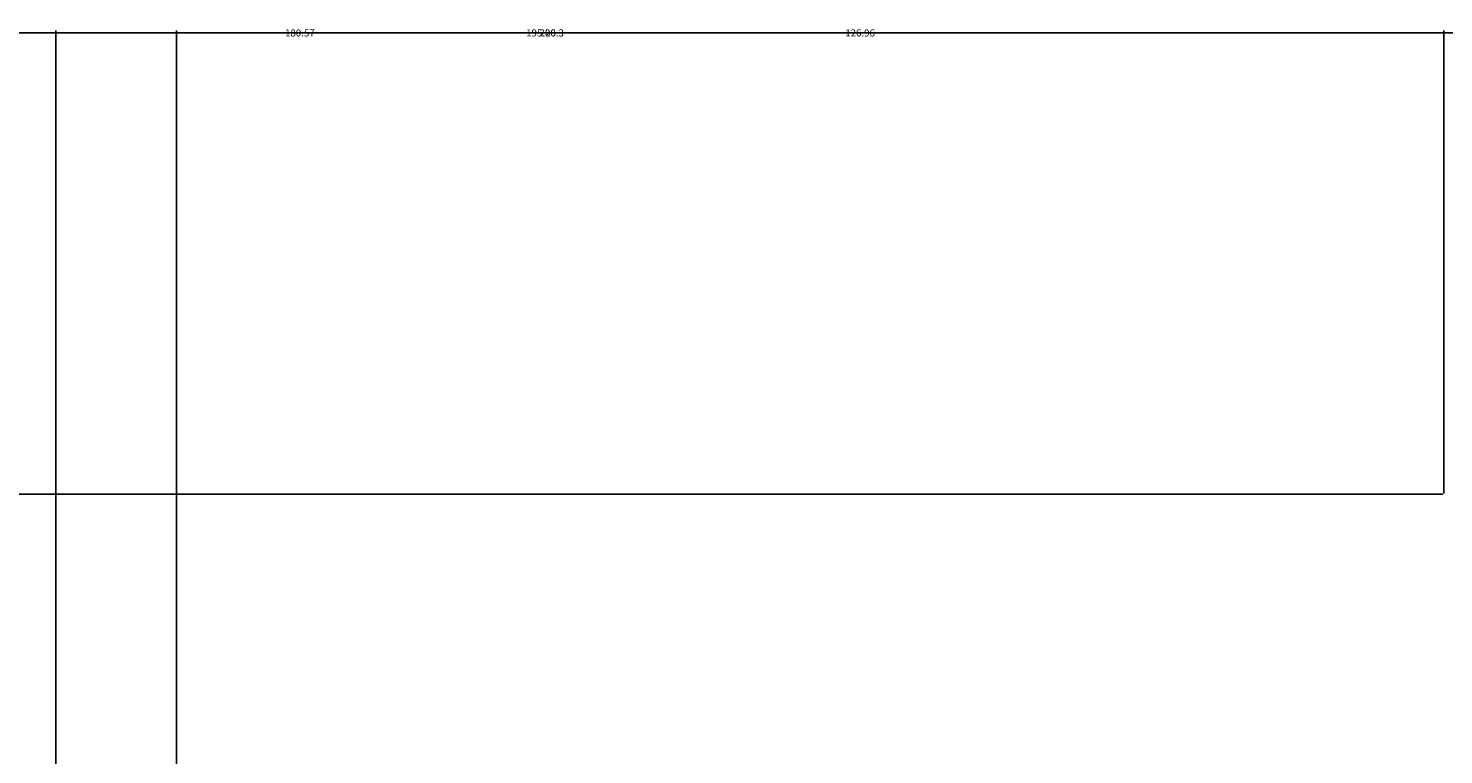
# Model space of a CAD drawing. Units: inches. Extents: x -26 to 776, y -22 to 650.
# Tile 32 of 62: x 80 to 192, y 593 to 650. Entities that reach past the tile are written whole.
import ezdxf

# ---------------------------------------------------------------- set-up
doc = ezdxf.new("R2010")
doc.units = ezdxf.units.IN
doc.header["$MEASUREMENT"] = 0
doc.layers.add('A-ANNO-DIMS', color=2, linetype='Continuous', lineweight=18)
doc.styles.get("Standard").update_dxf_attribs({"font": 'arial.ttf'})
doc.dimstyles.get("Standard").update_dxf_attribs({"dimtxt": 0.5625, "dimasz": 0.18, "dimexe": 0.18, "dimexo": 0.0625, "dimgap": 0.09, "dimtad": 0, "dimtih": 1, "dimtoh": 1, "dimdec": 4, "dimzin": 0, "dimdsep": 46, "dimlunit": 4, "dimtxsty": 'Standard', "dimcen": 0.09, "dimadec": 0, "dimazin": 0, "dimtfac": 1, "dimtdec": 4, "dimtofl": 0, "dimtmove": 0, "dimatfit": 3, "dimfxl": 1, "dimtolj": 1, "dimtzin": 0, "dimarcsym": 0})

# ---------------------------------------------------------------- blocks, each defined once
blk = doc.blocks.new('*D14')
at = {"layer": 'A-ANNO-DIMS', "color": 0, "lineweight": -2, "transparency": 16777216}
for p, q in [((191.62, 613.27), (-25.48, 613.27)), ((-25.3, 613.09), (-25.3, 314.75)), ((-25.3, 15.66), (-25.3, 314)), ((11.04, 15.48), (-25.48, 15.48))]:
    blk.add_line(p, q, dxfattribs=at)
at = {"layer": 'A-ANNO-DIMS', "color": 0, "transparency": 16777216}
for points in [[(-25.33, 613.09), (-25.27, 613.09), (-25.3, 613.27)], [(-25.33, 15.66), (-25.27, 15.66), (-25.3, 15.48)]]:
    blk.add_solid(points, dxfattribs=at)
at = {"layer": 'Defpoints', "color": 0, "transparency": 16777216}
for p in [(-25.3, 613.27), (191.68, 613.27), (11.11, 15.48)]:
    blk.add_point(p, dxfattribs=at)
at = {"layer": 'A-ANNO-DIMS', "color": 0, "transparency": 16777216, "insert": (-25.3, 314.38), "char_height": 0.562, "attachment_point": 5}
blk.add_mtext('\\A1;597.8', dxfattribs=at)
blk = doc.blocks.new('*D15')
at = {"layer": 'A-ANNO-DIMS', "color": 0, "lineweight": -2, "transparency": 16777216}
for p, q in [((11.11, 491.49), (11.11, 649.86)), ((11.29, 649.68), (120.22, 649.68)), ((231.24, 649.68), (122.31, 649.68)), ((231.42, 491.49), (231.42, 649.86))]:
    blk.add_line(p, q, dxfattribs=at)
at = {"layer": 'A-ANNO-DIMS', "color": 0, "transparency": 16777216}
for points in [[(11.29, 649.71), (11.29, 649.65), (11.11, 649.68)], [(231.24, 649.71), (231.24, 649.65), (231.42, 649.68)]]:
    blk.add_solid(points, dxfattribs=at)
at = {"layer": 'Defpoints', "color": 0, "transparency": 16777216}
for p in [(231.42, 649.68), (11.11, 491.43), (231.42, 491.43)]:
    blk.add_point(p, dxfattribs=at)
at = {"layer": 'A-ANNO-DIMS', "color": 0, "transparency": 16777216, "insert": (121.27, 649.68), "char_height": 0.562, "attachment_point": 5}
blk.add_mtext('\\A1;220.3', dxfattribs=at)
blk = doc.blocks.new('*D17')
at = {"layer": 'A-ANNO-DIMS', "color": 0, "lineweight": -2, "transparency": 16777216}
for p, q in [((11.11, 491.49), (11.11, 649.86)), ((11.29, 649.68), (100.16, 649.68)), ((191.5, 649.68), (102.62, 649.68)), ((191.68, 613.33), (191.68, 649.86))]:
    blk.add_line(p, q, dxfattribs=at)
at = {"layer": 'A-ANNO-DIMS', "color": 0, "transparency": 16777216}
for points in [[(11.29, 649.71), (11.29, 649.65), (11.11, 649.68)], [(191.5, 649.71), (191.5, 649.65), (191.68, 649.68)]]:
    blk.add_solid(points, dxfattribs=at)
at = {"layer": 'Defpoints', "color": 0, "transparency": 16777216}
for p in [(191.68, 649.68), (191.68, 613.27), (11.11, 491.43)]:
    blk.add_point(p, dxfattribs=at)
at = {"layer": 'A-ANNO-DIMS', "color": 0, "transparency": 16777216, "insert": (101.39, 649.68), "char_height": 0.562, "attachment_point": 5}
blk.add_mtext('\\A1;180.57', dxfattribs=at)
blk = doc.blocks.new('*D18')
at = {"layer": 'A-ANNO-DIMS', "color": 0, "lineweight": -2, "transparency": 16777216}
for p, q in [((191.68, 613.33), (191.68, 649.86)), ((191.86, 649.68), (273.36, 649.68)), ((356.89, 649.68), (275.38, 649.68)), ((357.07, 613.33), (357.07, 649.86))]:
    blk.add_line(p, q, dxfattribs=at)
at = {"layer": 'A-ANNO-DIMS', "color": 0, "transparency": 16777216}
for points in [[(191.86, 649.71), (191.86, 649.65), (191.68, 649.68)], [(356.89, 649.71), (356.89, 649.65), (357.07, 649.68)]]:
    blk.add_solid(points, dxfattribs=at)
at = {"layer": 'Defpoints', "color": 0, "transparency": 16777216}
for p in [(357.07, 649.68), (191.68, 613.27), (357.07, 613.27)]:
    blk.add_point(p, dxfattribs=at)
at = {"layer": 'A-ANNO-DIMS', "color": 0, "transparency": 16777216, "insert": (274.37, 649.68), "char_height": 0.562, "attachment_point": 5}
blk.add_mtext('\\A1;165.4', dxfattribs=at)
blk = doc.blocks.new('*D19')
at = {"layer": 'A-ANNO-DIMS', "color": 0, "lineweight": -2, "transparency": 16777216}
for p, q in [((191.62, 613.27), (-25.48, 613.27)), ((-25.3, 613.09), (-25.3, 552.73)), ((-25.3, 491.61), (-25.3, 551.97)), ((191.62, 491.43), (-25.48, 491.43))]:
    blk.add_line(p, q, dxfattribs=at)
at = {"layer": 'A-ANNO-DIMS', "color": 0, "transparency": 16777216}
for points in [[(-25.33, 613.09), (-25.27, 613.09), (-25.3, 613.27)], [(-25.33, 491.61), (-25.27, 491.61), (-25.3, 491.43)]]:
    blk.add_solid(points, dxfattribs=at)
at = {"layer": 'Defpoints', "color": 0, "transparency": 16777216}
for p in [(-25.3, 613.27), (191.68, 613.27), (191.68, 491.43)]:
    blk.add_point(p, dxfattribs=at)
at = {"layer": 'A-ANNO-DIMS', "color": 0, "transparency": 16777216, "insert": (-25.3, 552.35), "char_height": 0.562, "attachment_point": 5}
blk.add_mtext('\\A1;121.84', dxfattribs=at)
blk = doc.blocks.new('*D22')
at = {"layer": 'A-ANNO-DIMS', "color": 0, "lineweight": -2, "transparency": 16777216}
for p, q in [((22.89, 15.33), (22.89, 649.86)), ((23.07, 649.68), (119.19, 649.68)), ((217.77, 649.68), (121.65, 649.68)), ((217.95, 15.54), (217.95, 649.86))]:
    blk.add_line(p, q, dxfattribs=at)
at = {"layer": 'A-ANNO-DIMS', "color": 0, "transparency": 16777216}
for points in [[(23.07, 649.71), (23.07, 649.65), (22.89, 649.68)], [(217.77, 649.71), (217.77, 649.65), (217.95, 649.68)]]:
    blk.add_solid(points, dxfattribs=at)
at = {"layer": 'Defpoints', "color": 0, "transparency": 16777216}
for p in [(217.95, 649.68), (22.89, 15.27), (217.95, 15.48)]:
    blk.add_point(p, dxfattribs=at)
at = {"layer": 'A-ANNO-DIMS', "color": 0, "transparency": 16777216, "insert": (120.42, 649.68), "char_height": 0.562, "attachment_point": 5}
blk.add_mtext('\\A1;195.06', dxfattribs=at)
blk = doc.blocks.new('*D25')
at = {"layer": 'A-ANNO-DIMS', "color": 0, "lineweight": -2, "transparency": 16777216}
for p, q in [((11.11, 221.7), (11.11, 649.86)), ((11.29, 649.68), (50.34, 649.68)), ((91.46, 649.68), (52.41, 649.68)), ((91.64, 271.37), (91.64, 649.86))]:
    blk.add_line(p, q, dxfattribs=at)
at = {"layer": 'A-ANNO-DIMS', "color": 0, "transparency": 16777216}
for points in [[(11.29, 649.71), (11.29, 649.65), (11.11, 649.68)], [(91.46, 649.71), (91.46, 649.65), (91.64, 649.68)]]:
    blk.add_solid(points, dxfattribs=at)
at = {"layer": 'Defpoints', "color": 0, "transparency": 16777216}
for p in [(91.64, 649.68), (91.64, 271.31), (11.11, 221.64)]:
    blk.add_point(p, dxfattribs=at)
at = {"layer": 'A-ANNO-DIMS', "color": 0, "transparency": 16777216, "insert": (51.38, 649.68), "char_height": 0.562, "attachment_point": 5}
blk.add_mtext('\\A1;80.54', dxfattribs=at)
blk = doc.blocks.new('*D35')
at = {"layer": 'A-ANNO-DIMS', "color": 0, "lineweight": -2, "transparency": 16777216}
for p, q in [((82.13, 420.34), (82.13, 649.86)), ((82.31, 649.68), (144.38, 649.68)), ((208.91, 649.68), (146.84, 649.68)), ((209.09, 420.34), (209.09, 649.86))]:
    blk.add_line(p, q, dxfattribs=at)
at = {"layer": 'A-ANNO-DIMS', "color": 0, "transparency": 16777216}
for points in [[(82.31, 649.71), (82.31, 649.65), (82.13, 649.68)], [(208.91, 649.71), (208.91, 649.65), (209.09, 649.68)]]:
    blk.add_solid(points, dxfattribs=at)
at = {"layer": 'Defpoints', "color": 0, "transparency": 16777216}
for p in [(209.09, 649.68), (82.13, 420.28), (209.09, 420.28)]:
    blk.add_point(p, dxfattribs=at)
at = {"layer": 'A-ANNO-DIMS', "color": 0, "transparency": 16777216, "insert": (145.61, 649.68), "char_height": 0.562, "attachment_point": 5}
blk.add_mtext('\\A1;126.96', dxfattribs=at)

msp = doc.modelspace()

# ---------------------------------------------------------------- dimensions: what is measured, and where the dimension line sits
at = {"layer": 'A-ANNO-DIMS'}
for base, p1, p2, override, picture, middle in [((231.4249, 649.6763), (11.1074, 491.4269), (231.4249, 491.4269), {"dimdec": 1, "dimlfac": 1, "dimrnd": 0, "dimzin": 0, "dimdsep": 46, "dimlunit": 2}, '*D15', (121.2661, 649.6763)), ((191.6782, 649.6763), (11.1074, 491.4269), (191.6782, 613.2713), {"dimdec": 2, "dimlfac": 1, "dimrnd": 0, "dimzin": 0, "dimdsep": 46, "dimlunit": 2}, '*D17', (101.3928, 649.6763)), ((91.6448, 649.6763), (11.1074, 221.6413), (91.6448, 271.3091), {"dimdec": 2, "dimlfac": 1, "dimrnd": 0, "dimzin": 0, "dimdsep": 46, "dimlunit": 2}, '*D25', (51.3761, 649.6763)), ((217.9529, 649.6763), (22.8891, 15.2701), (217.9529, 15.4824), {"dimdec": 2, "dimlfac": 1, "dimrnd": 0, "dimzin": 0, "dimdsep": 46, "dimlunit": 2}, '*D22', (120.421, 649.6763)), ((209.091, 649.6763), (82.134, 420.2783), (209.091, 420.2783), {"dimdec": 2, "dimlfac": 1, "dimrnd": 0, "dimzin": 0, "dimdsep": 46, "dimlunit": 2}, '*D35', (145.6125, 649.6763)), ((357.0669, 649.6763), (191.6782, 613.2713), (357.0669, 613.2713), {"dimdec": 1, "dimlfac": 1, "dimrnd": 0, "dimzin": 0, "dimdsep": 46, "dimlunit": 2}, '*D18', (274.3725, 649.6763))]:
    dim = msp.add_linear_dim(base=base, p1=p1, p2=p2, dimstyle='Standard', override=override, dxfattribs=at)
    dim.commit()
    dim.dimension.update_dxf_attribs({"geometry": picture, "text_midpoint": middle})
for p1, override, picture, middle in [((191.6782, 491.4269), {"dimdec": 2, "dimlfac": 1, "dimrnd": 0, "dimzin": 0, "dimdsep": 46, "dimlunit": 2}, '*D19', (-25.2976, 552.3491)), ((11.1074, 15.4824), {"dimdec": 1, "dimlfac": 1, "dimrnd": 0, "dimzin": 0, "dimdsep": 46, "dimlunit": 2}, '*D14', (-25.2976, 314.3769))]:
    dim = msp.add_linear_dim(base=(-25.2976, 613.2713), p1=p1, p2=(191.6782, 613.2713), angle=90, dimstyle='Standard', override=override, dxfattribs=at)
    dim.commit()
    dim.dimension.update_dxf_attribs({"geometry": picture, "text_midpoint": middle})

doc.saveas('drawing.dxf')
